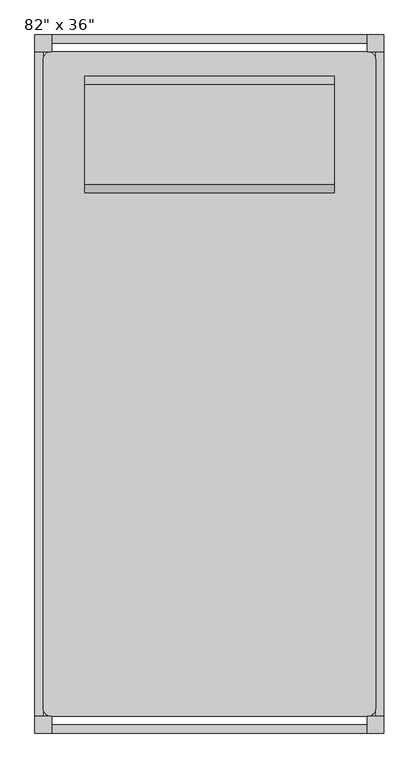
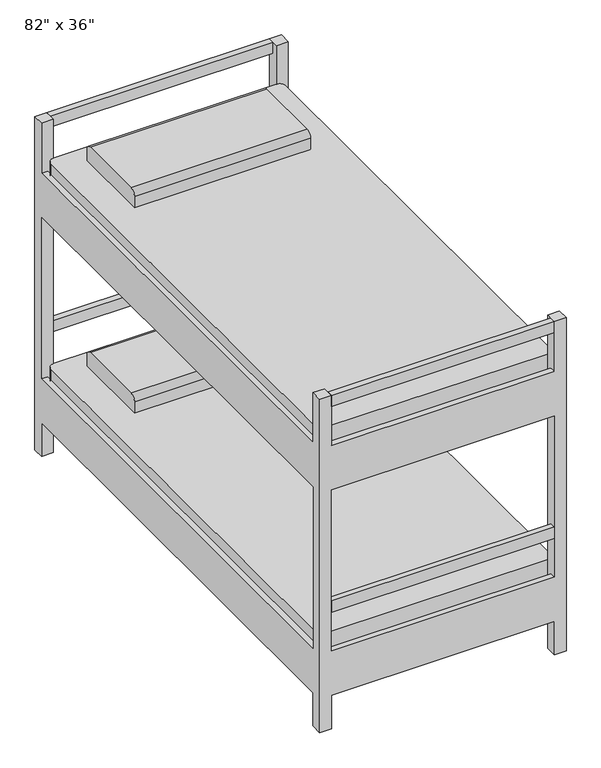
"""IFC4 building model written with IfcOpenShell, lengths in millimetres: furniture geometry."""

from ifc_helpers import new_model, si_unit, point, frame, frame_2d, origin, place, context, project, spatial, polyline, circle_curve, trimmed, segment, composite_curve, outline, extrude, faceted_brep, source, transform, mapped, element, save


def furniture_5816963c(model_context):
    return source(origin(), model_context, "Body", "SolidModel", [
        faceted_brep([(-74.1180328, -1457.7934426, 1295.4), (891.0819672, -1457.7934426, 1295.4), (891.0819672, -1432.3934426, 1295.4), (-74.1180328, -1432.3934426, 1295.4), (941.8819672, -1406.9934426, 1295.4), (941.8819672, 625.0065574, 1295.4), (916.4819672, 625.0065574, 1295.4), (916.4819672, -1406.9934426, 1295.4), (891.0819672, 675.8065574, 1295.4), (-74.1180328, 675.8065574, 1295.4), (-74.1180328, 650.4065574, 1295.4), (891.0819672, 650.4065574, 1295.4), (-124.9180328, 625.0065574, 1295.4), (-124.9180328, -1406.9934426, 1295.4), (-99.5180328, -1406.9934426, 1295.4), (-99.5180328, 625.0065574, 1295.4), (-124.9180328, -1406.9934426, 1092.2), (-124.9180328, 625.0065574, 1092.2), (-99.5180328, 625.0065574, 1092.2), (-99.5180328, -1406.9934426, 1092.2), (-74.1180328, 675.8065574, 1092.2), (891.0819672, 675.8065574, 1092.2), (891.0819672, 650.4065574, 1092.2), (-74.1180328, 650.4065574, 1092.2), (941.8819672, 625.0065574, 1092.2), (941.8819672, -1406.9934426, 1092.2), (916.4819672, -1406.9934426, 1092.2), (916.4819672, 625.0065574, 1092.2), (891.0819672, -1457.7934426, 1092.2), (-74.1180328, -1457.7934426, 1092.2), (-74.1180328, -1432.3934426, 1092.2), (891.0819672, -1432.3934426, 1092.2), (-74.1180328, -1457.7934426, 1524.0), (-124.9180328, -1457.7934426, 1524.0), (-124.9180328, -1457.7934426, 0.0), (-74.1180328, -1457.7934426, 0.0), (-74.1180328, -1457.7934426, 152.4), (891.0819672, -1457.7934426, 152.4), (891.0819672, -1457.7934426, 0.0), (941.8819672, -1457.7934426, 0.0), (941.8819672, -1457.7934426, 1524.0), (891.0819672, -1457.7934426, 1524.0), (891.0819672, -1457.7934426, 355.6), (-74.1180328, -1457.7934426, 355.6), (941.8819672, 675.8065574, 1524.0), (941.8819672, 625.0065574, 1524.0), (941.8819672, -1406.9934426, 1524.0), (941.8819672, -1406.9934426, 0.0), (941.8819672, -1406.9934426, 152.4), (941.8819672, 625.0065574, 152.4), (941.8819672, 625.0065574, 0.0), (941.8819672, 675.8065574, 0.0), (941.8819672, 625.0065574, 355.6), (941.8819672, -1406.9934426, 355.6), (-124.9180328, 675.8065574, 1524.0), (-74.1180328, 675.8065574, 1524.0), (891.0819672, 675.8065574, 1524.0), (891.0819672, 675.8065574, 0.0), (891.0819672, 675.8065574, 152.4), (-74.1180328, 675.8065574, 152.4), (-74.1180328, 675.8065574, 0.0), (-124.9180328, 675.8065574, 0.0), (-74.1180328, 675.8065574, 355.6), (891.0819672, 675.8065574, 355.6), (-124.9180328, 625.0065574, 1524.0), (-124.9180328, 625.0065574, 0.0), (-124.9180328, 625.0065574, 152.4), (-124.9180328, -1406.9934426, 152.4), (-124.9180328, -1406.9934426, 0.0), (-124.9180328, -1406.9934426, 1524.0), (-124.9180328, -1406.9934426, 355.6), (-124.9180328, 625.0065574, 355.6), (891.0819672, -1406.9934426, 1524.0), (-74.1180328, 625.0065574, 1524.0), (891.0819672, 625.0065574, 1524.0), (-74.1180328, -1406.9934426, 1524.0), (-74.1180328, -1406.9934426, 0.0), (891.0819672, 625.0065574, 0.0), (-74.1180328, 625.0065574, 0.0), (891.0819672, -1406.9934426, 0.0), (-99.5180328, 625.0065574, 355.6), (-99.5180328, 625.0065574, 152.4), (-74.1180328, 650.4065574, 152.4), (-74.1180328, 650.4065574, 355.6), (891.0819672, 650.4065574, 355.6), (891.0819672, 650.4065574, 152.4), (916.4819672, 625.0065574, 152.4), (916.4819672, 625.0065574, 355.6), (-74.1180328, -1432.3934426, 355.6), (-74.1180328, -1432.3934426, 152.4), (-99.5180328, -1406.9934426, 152.4), (-99.5180328, -1406.9934426, 355.6), (916.4819672, -1406.9934426, 355.6), (916.4819672, -1406.9934426, 152.4), (891.0819672, -1432.3934426, 152.4), (891.0819672, -1432.3934426, 355.6)], [[[0, 1, 2, 3]], [[4, 5, 6, 7]], [[8, 9, 10, 11]], [[12, 13, 14, 15]], [[16, 17, 18, 19]], [[20, 21, 22, 23]], [[24, 25, 26, 27]], [[28, 29, 30, 31]], [[32, 33, 34, 35, 36, 37, 38, 39, 40, 41, 1, 0], [28, 42, 43, 29]], [[44, 45, 5, 4, 46, 40, 39, 47, 48, 49, 50, 51], [24, 52, 53, 25]], [[54, 55, 9, 8, 56, 44, 51, 57, 58, 59, 60, 61], [20, 62, 63, 21]], [[64, 54, 61, 65, 66, 67, 68, 34, 33, 69, 13, 12], [16, 70, 71, 17]], [[11, 10, 23, 22]], [[7, 6, 27, 26]], [[3, 2, 31, 30]], [[15, 14, 19, 18]], [[41, 40, 46, 72]], [[55, 54, 64, 73]], [[56, 74, 45, 44]], [[32, 75, 69, 33]], [[35, 34, 68, 76]], [[57, 51, 50, 77]], [[60, 78, 65, 61]], [[38, 79, 47, 39]], [[73, 64, 12, 15, 18, 17, 71, 80, 81, 66, 65, 78]], [[55, 73, 78, 60, 59, 82, 83, 62, 20, 23, 10, 9]], [[74, 56, 8, 11, 22, 21, 63, 84, 85, 58, 57, 77]], [[45, 74, 77, 50, 49, 86, 87, 52, 24, 27, 6, 5]], [[75, 32, 0, 3, 30, 29, 43, 88, 89, 36, 35, 76]], [[69, 75, 76, 68, 67, 90, 91, 70, 16, 19, 14, 13]], [[72, 46, 4, 7, 26, 25, 53, 92, 93, 48, 47, 79]], [[41, 72, 79, 38, 37, 94, 95, 42, 28, 31, 2, 1]], [[43, 42, 95, 88]], [[53, 52, 87, 92]], [[63, 62, 83, 84]], [[71, 70, 91, 80]], [[37, 36, 89, 94]], [[49, 48, 93, 86]], [[59, 58, 85, 82]], [[67, 66, 81, 90]], [[92, 87, 86, 93]], [[88, 95, 94, 89]], [[80, 91, 90, 81]], [[84, 83, 82, 85]]]),
        extrude(outline(composite_curve([segment(polyline([(548.8065574, 406.4), (193.2065574, 406.4), (193.2065574, 457.2)]), True, "CONTINUOUS"), segment(trimmed(circle_curve(frame_2d((218.6065574, 457.2)), 25.4), [point((193.2065574, 457.2))], [point((218.6065574, 482.6))], False, "CARTESIAN"), True, "CONTINUOUS"), segment(polyline([(218.6065574, 482.6), (523.4065574, 482.6)]), True, "CONTINUOUS"), segment(trimmed(circle_curve(frame_2d((523.4065574, 457.2)), 25.4), [point((523.4065574, 482.6))], [point((548.8065574, 457.2))], False, "CARTESIAN"), True, "CONTINUOUS"), segment(polyline([(548.8065574, 457.2), (548.8065574, 406.4)]), True, "CONTINUOUS")], self_intersect=False)), frame((27.4819672, 0.0, 0.0), z_axis=(1.0, 0.0, 0.0), x_axis=(0.0, 1.0, 0.0)), (0.0, 0.0, 1.0), 762.0),
        extrude(outline(composite_curve([segment(polyline([(548.8065574, 1346.2), (193.2065574, 1346.2), (193.2065574, 1397.0)]), True, "CONTINUOUS"), segment(trimmed(circle_curve(frame_2d((218.6065574, 1397.0)), 25.4), [point((193.2065574, 1397.0))], [point((218.6065574, 1422.4))], False, "CARTESIAN"), True, "CONTINUOUS"), segment(polyline([(218.6065574, 1422.4), (523.4065574, 1422.4)]), True, "CONTINUOUS"), segment(trimmed(circle_curve(frame_2d((523.4065574, 1397.0)), 25.4), [point((523.4065574, 1422.4))], [point((548.8065574, 1397.0))], False, "CARTESIAN"), True, "CONTINUOUS"), segment(polyline([(548.8065574, 1397.0), (548.8065574, 1346.2)]), True, "CONTINUOUS")], self_intersect=False)), frame((27.4819672, 0.0, 0.0), z_axis=(1.0, 0.0, 0.0), x_axis=(0.0, 1.0, 0.0)), (0.0, 0.0, 1.0), 762.0),
        extrude(outline(polyline([(891.0819672, -1457.7934426), (-74.1180328, -1457.7934426), (-74.1180328, -1432.3934426), (891.0819672, -1432.3934426), (891.0819672, -1457.7934426)])), frame((0.0, 0.0, 533.4), z_axis=(0.0, 0.0, 1.0), x_axis=(1.0, 0.0, 0.0)), (0.0, 0.0, 1.0), 50.8),
        extrude(outline(polyline([(891.0819672, 675.8065574), (891.0819672, 650.4065574), (-74.1180328, 650.4065574), (-74.1180328, 675.8065574), (891.0819672, 675.8065574)])), frame((0.0, 0.0, 533.4), z_axis=(0.0, 0.0, 1.0), x_axis=(1.0, 0.0, 0.0)), (0.0, 0.0, 1.0), 50.8),
        extrude(outline(polyline([(891.0819672, 675.8065574), (891.0819672, 650.4065574), (-74.1180328, 650.4065574), (-74.1180328, 675.8065574), (891.0819672, 675.8065574)])), frame((0.0, 0.0, 1473.2), z_axis=(0.0, 0.0, 1.0), x_axis=(1.0, 0.0, 0.0)), (0.0, 0.0, 1.0), 50.8),
        extrude(outline(polyline([(891.0819672, -1457.7934426), (-74.1180328, -1457.7934426), (-74.1180328, -1432.3934426), (891.0819672, -1432.3934426), (891.0819672, -1457.7934426)])), frame((0.0, 0.0, 1473.2), z_axis=(0.0, 0.0, 1.0), x_axis=(1.0, 0.0, 0.0)), (0.0, 0.0, 1.0), 50.8),
        extrude(outline(composite_curve([segment(trimmed(circle_curve(frame_2d((891.0819672, 599.6065574)), 25.4), [point((891.0819672, 625.0065574))], [point((916.4819672, 599.6065574))], False, "CARTESIAN"), True, "CONTINUOUS"), segment(polyline([(916.4819672, 599.6065574), (916.4819672, -1381.5934426)]), True, "CONTINUOUS"), segment(trimmed(circle_curve(frame_2d((891.0819672, -1381.5934426)), 25.4), [point((916.4819672, -1381.5934426))], [point((891.0819672, -1406.9934426))], False, "CARTESIAN"), True, "CONTINUOUS"), segment(polyline([(891.0819672, -1406.9934426), (-74.1180328, -1406.9934426)]), True, "CONTINUOUS"), segment(trimmed(circle_curve(frame_2d((-74.1180328, -1381.5934426)), 25.4), [point((-74.1180328, -1406.9934426))], [point((-99.5180328, -1381.5934426))], False, "CARTESIAN"), True, "CONTINUOUS"), segment(polyline([(-99.5180328, -1381.5934426), (-99.5180328, 599.6065574)]), True, "CONTINUOUS"), segment(trimmed(circle_curve(frame_2d((-74.1180328, 599.6065574)), 25.4), [point((-99.5180328, 599.6065574))], [point((-74.1180328, 625.0065574))], False, "CARTESIAN"), True, "CONTINUOUS"), segment(polyline([(-74.1180328, 625.0065574), (891.0819672, 625.0065574)]), True, "CONTINUOUS")], self_intersect=False)), frame((0.0, 0.0, 1143.0), z_axis=(0.0, 0.0, 1.0), x_axis=(1.0, 0.0, 0.0)), (0.0, 0.0, 1.0), 203.2),
        extrude(outline(composite_curve([segment(trimmed(circle_curve(frame_2d((891.0819672, 599.6065574)), 25.4), [point((891.0819672, 625.0065574))], [point((916.4819672, 599.6065574))], False, "CARTESIAN"), True, "CONTINUOUS"), segment(polyline([(916.4819672, 599.6065574), (916.4819672, -1381.5934426)]), True, "CONTINUOUS"), segment(trimmed(circle_curve(frame_2d((891.0819672, -1381.5934426)), 25.4), [point((916.4819672, -1381.5934426))], [point((891.0819672, -1406.9934426))], False, "CARTESIAN"), True, "CONTINUOUS"), segment(polyline([(891.0819672, -1406.9934426), (-74.1180328, -1406.9934426)]), True, "CONTINUOUS"), segment(trimmed(circle_curve(frame_2d((-74.1180328, -1381.5934426)), 25.4), [point((-74.1180328, -1406.9934426))], [point((-99.5180328, -1381.5934426))], False, "CARTESIAN"), True, "CONTINUOUS"), segment(polyline([(-99.5180328, -1381.5934426), (-99.5180328, 599.6065574)]), True, "CONTINUOUS"), segment(trimmed(circle_curve(frame_2d((-74.1180328, 599.6065574)), 25.4), [point((-99.5180328, 599.6065574))], [point((-74.1180328, 625.0065574))], False, "CARTESIAN"), True, "CONTINUOUS"), segment(polyline([(-74.1180328, 625.0065574), (891.0819672, 625.0065574)]), True, "CONTINUOUS")], self_intersect=False)), frame((0.0, 0.0, 203.2), z_axis=(0.0, 0.0, 1.0), x_axis=(1.0, 0.0, 0.0)), (0.0, 0.0, 1.0), 203.2),
    ])


if __name__ == "__main__":
    model = new_model("IFC4")
    model_context = context("Model", 3, world=origin())
    ifc_project = project(units=[si_unit("LENGTHUNIT", "METRE", prefix="MILLI")], contexts=[model_context])
    site = spatial("IfcSite", under=ifc_project)
    building = spatial("IfcBuilding", under=site)
    placement = place(None, origin())
    furniture_shape = furniture_5816963c(model_context)
    element("IfcFurniture", 1, ObjectType="82\" x 36\"", at=placement, inside=building, context=model_context, shape_type="MappedRepresentation", body=[
        mapped(furniture_shape, transform((0.0, 0.0, 0.0), x_axis=(1.0, 0.0, 0.0), y_axis=(0.0, 1.0, 0.0), z_axis=(0.0, 0.0, 1.0))),
    ])
    save(model, "model.ifc")

# Revit data of these elements
# Type "82\" x 36\""
#   Assembly Code = "E2020200"
#   Height = 5' - 0"
#   Length = 7' - 0"
#   Width = 3' - 6"
#   Frame Material = Birch
#   Mattress Material = Linen, White
#   Default Elevation = 0
# Element 1 (IfcFurniture, "82\" x 36\"")
#   Materials on its faces: "Birch", "Linen, White"
# Materials
#   "Birch": class "Wood", colour RGB 224 178 126, transparency 0, Description = "Betula Alleghaniensis", Cost = 0
#   "Linen, White": class "Textile", colour RGB 247 247 239, transparency 0, Description = "Linen, white", Cost = 0
